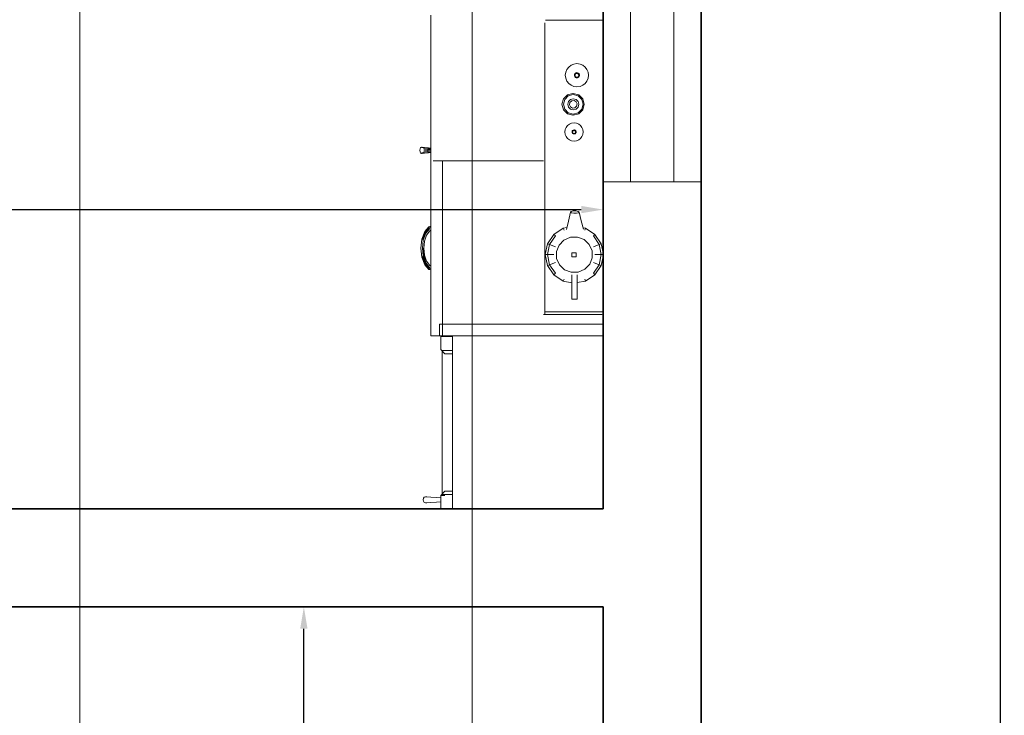
# Model space of a CAD drawing. Units: feet. Extents: x -297 to 770, y -228 to 625.
# Tile 9 of 14: x 680 to 770, y 95 to 158. Entities that reach past the tile are written whole.
import ezdxf

# ---------------------------------------------------------------- set-up
doc = ezdxf.new("R2010")
doc.units = ezdxf.units.FT
doc.header["$MEASUREMENT"] = 0
for name, color, linetype, lineweight in [('A-ANNO-DIMS', 2, 'Continuous', 18), ('A-EQPM', 8, 'Continuous', 13), ('A-FLOR-CASE', 8, 'Continuous', 18), ('A-WALL', 7, 'Continuous', 35), ('windows', 30, 'Continuous', 18)]:
    doc.layers.add(name, color=color, linetype=linetype, lineweight=lineweight)
doc.styles.get("Standard").update_dxf_attribs({"font": 'arial.ttf'})
doc.dimstyles.get("Standard").update_dxf_attribs({"dimtxt": 3, "dimasz": 2, "dimexe": 0.18, "dimexo": 0.0625, "dimgap": 0.09, "dimtad": 1, "dimtoh": 1, "dimdec": 1, "dimzin": 0, "dimdsep": 46, "dimlunit": 3, "dimtxsty": 'Standard', "dimcen": 0, "dimclre": 256, "dimadec": 0, "dimazin": 0, "dimtfac": 1, "dimtdec": 1, "dimtofl": 0, "dimtmove": 0, "dimatfit": 3, "dimfxl": 1, "dimtolj": 1, "dimtzin": 0, "dimlwe": -1, "dimarcsym": 0})

# ---------------------------------------------------------------- blocks, each defined once
blk = doc.blocks.new('WIN-5FT')
for p, q in [((60, 6.5), (0, 6.5)), ((60, 2.5), (0, 2.5))]:
    blk.add_line(p, q)
blk.add_lwpolyline([(60, 0), (60, 9), (0, 9), (0, 0)], close=True)
blk = doc.blocks.new('*D44')
at = {"layer": 'A-ANNO-DIMS', "transparency": 16777216}
for p, q in [((742.218, 306.963), (769.785, 306.963)), ((742.218, -200.037), (769.785, -200.037))]:
    blk.add_line(p, q, dxfattribs=at)
at = {"layer": 'A-ANNO-DIMS', "color": 0, "lineweight": -2, "transparency": 16777216}
blk.add_line((769.605, -198.037), (769.605, 304.963), dxfattribs=at)
at = {"layer": 'A-ANNO-DIMS', "color": 0, "transparency": 16777216}
for points in [[(769.272, 304.963), (769.939, 304.963), (769.605, 306.963)], [(769.272, -198.037), (769.939, -198.037), (769.605, -200.037)]]:
    blk.add_solid(points, dxfattribs=at)
at = {"layer": 'Defpoints', "color": 0, "transparency": 16777216}
for p in [(742.155, 306.963), (769.605, 306.963), (742.155, -200.037)]:
    blk.add_point(p, dxfattribs=at)
at = {"layer": 'A-ANNO-DIMS', "color": 0, "transparency": 16777216, "insert": (767.984, 53.463), "char_height": 3, "attachment_point": 5, "rotation": 90}
blk.add_mtext('\\A1;507', dxfattribs=at)
blk = doc.blocks.new('*D55')
at = {"layer": 'A-ANNO-DIMS', "transparency": 16777216}
for p, q in [((733.093, 104.463), (705.525, 104.463)), ((733.093, 45.463), (705.525, 45.463))]:
    blk.add_line(p, q, dxfattribs=at)
at = {"layer": 'A-ANNO-DIMS', "color": 0, "lineweight": -2, "transparency": 16777216}
blk.add_line((705.705, 47.463), (705.705, 102.463), dxfattribs=at)
at = {"layer": 'A-ANNO-DIMS', "color": 0, "transparency": 16777216}
for points in [[(705.372, 102.463), (706.039, 102.463), (705.705, 104.463)], [(705.372, 47.463), (706.039, 47.463), (705.705, 45.463)]]:
    blk.add_solid(points, dxfattribs=at)
at = {"layer": 'Defpoints', "color": 0, "transparency": 16777216}
for p in [(705.705, 104.463), (733.155, 104.463), (733.155, 45.463)]:
    blk.add_point(p, dxfattribs=at)
at = {"layer": 'A-ANNO-DIMS', "color": 0, "transparency": 16777216, "insert": (704.084, 74.963), "char_height": 3, "attachment_point": 5, "rotation": 90}
blk.add_mtext('\\A1;59', dxfattribs=at)
blk = doc.blocks.new('*D68')
at = {"layer": 'A-ANNO-DIMS', "transparency": 16777216}
for p, q in [((685.155, 306.9), (685.155, -227.667)), ((721.155, 306.9), (721.155, -227.667))]:
    blk.add_line(p, q, dxfattribs=at)
at = {"layer": 'A-ANNO-DIMS', "color": 0, "lineweight": -2, "transparency": 16777216}
blk.add_line((687.155, -227.487), (719.155, -227.487), dxfattribs=at)
at = {"layer": 'A-ANNO-DIMS', "color": 0, "transparency": 16777216}
for points in [[(687.155, -227.154), (687.155, -227.821), (685.155, -227.487)], [(719.155, -227.154), (719.155, -227.821), (721.155, -227.487)]]:
    blk.add_solid(points, dxfattribs=at)
at = {"layer": 'Defpoints', "color": 0, "transparency": 16777216}
for p in [(685.155, 306.963), (721.155, 306.963), (721.155, -227.487)]:
    blk.add_point(p, dxfattribs=at)
at = {"layer": 'A-ANNO-DIMS', "color": 0, "transparency": 16777216, "insert": (703.155, -225.865), "char_height": 3, "attachment_point": 5}
blk.add_mtext('\\A1;36', dxfattribs=at)
blk = doc.blocks.new('*D84')
at = {"layer": 'A-ANNO-DIMS', "transparency": 16777216}
for p, q in [((592.155, 113.525), (592.155, 141.093)), ((733.155, 113.525), (733.155, 141.093))]:
    blk.add_line(p, q, dxfattribs=at)
at = {"layer": 'A-ANNO-DIMS', "color": 0, "lineweight": -2, "transparency": 16777216}
blk.add_line((594.155, 140.913), (731.155, 140.913), dxfattribs=at)
at = {"layer": 'A-ANNO-DIMS', "color": 0, "transparency": 16777216}
for points in [[(594.155, 141.246), (594.155, 140.579), (592.155, 140.913)], [(731.155, 141.246), (731.155, 140.579), (733.155, 140.913)]]:
    blk.add_solid(points, dxfattribs=at)
at = {"layer": 'Defpoints', "color": 0, "transparency": 16777216}
for p in [(733.155, 140.913), (592.155, 113.463), (733.155, 113.463)]:
    blk.add_point(p, dxfattribs=at)
at = {"layer": 'A-ANNO-DIMS', "color": 0, "transparency": 16777216, "insert": (662.655, 142.509), "char_height": 3, "attachment_point": 5}
blk.add_mtext('\\A1;141', dxfattribs=at)

msp = doc.modelspace()

# ---------------------------------------------------------------- linework, layer by layer
at = {"layer": 'A-EQPM'}
for p, q in [((727.797, 131.305), (727.797, 158.049)), ((729.832, 153.777), (729.724, 153.523)), ((729.999, 153.993), (729.832, 153.777)), ((730.215, 154.16), (729.999, 153.993)), ((730.47, 154.268), (730.215, 154.16)), ((730.753, 154.306), (730.47, 154.268)), ((731.036, 154.268), (730.753, 154.306)), ((731.291, 154.16), (731.036, 154.268)), ((731.507, 153.993), (731.291, 154.16)), ((731.674, 153.777), (731.507, 153.993)), ((731.781, 153.523), (731.674, 153.777)), ((729.724, 153.523), (729.686, 153.239)), ((729.686, 153.239), (729.724, 152.956)), ((729.724, 152.956), (729.832, 152.701)), ((729.832, 152.701), (729.999, 152.485)), ((730.526, 153.302), (730.517, 153.239)), ((730.517, 153.239), (730.526, 153.177)), ((730.55, 153.358), (730.526, 153.302)), ((730.526, 153.177), (730.55, 153.12)), ((730.544, 153.297), (730.536, 153.239)), ((730.536, 153.239), (730.544, 153.181)), ((730.566, 153.349), (730.544, 153.297)), ((730.544, 153.181), (730.566, 153.13)), ((730.586, 153.406), (730.55, 153.358)), ((730.55, 153.12), (730.586, 153.073)), ((730.6, 153.393), (730.566, 153.349)), ((730.566, 153.13), (730.6, 153.086)), ((730.58, 153.276), (730.574, 153.229)), ((730.574, 153.229), (730.58, 153.181)), ((730.598, 153.319), (730.58, 153.276)), ((730.58, 153.181), (730.598, 153.139)), ((730.634, 153.443), (730.586, 153.406)), ((730.586, 153.073), (730.634, 153.036)), ((730.626, 153.355), (730.598, 153.319)), ((730.598, 153.139), (730.626, 153.102)), ((730.643, 153.426), (730.6, 153.393)), ((730.6, 153.086), (730.643, 153.052)), ((730.663, 153.383), (730.626, 153.355)), ((730.626, 153.102), (730.663, 153.074)), ((730.69, 153.466), (730.634, 153.443)), ((730.634, 153.036), (730.69, 153.012)), ((730.695, 153.448), (730.643, 153.426)), ((730.643, 153.052), (730.695, 153.03)), ((730.705, 153.401), (730.663, 153.383)), ((730.663, 153.074), (730.705, 153.056)), ((730.753, 153.475), (730.69, 153.466)), ((730.69, 153.012), (730.753, 153.003)), ((730.753, 153.456), (730.695, 153.448)), ((730.695, 153.03), (730.753, 153.022)), ((730.753, 153.408), (730.705, 153.401)), ((730.705, 153.056), (730.753, 153.05)), ((730.816, 153.466), (730.753, 153.475)), ((730.811, 153.448), (730.753, 153.456)), ((730.8, 153.401), (730.753, 153.408)), ((730.753, 153.05), (730.8, 153.056)), ((730.753, 153.022), (730.811, 153.03)), ((730.753, 153.003), (730.816, 153.012)), ((730.843, 153.383), (730.8, 153.401)), ((730.8, 153.056), (730.843, 153.074)), ((730.862, 153.426), (730.811, 153.448)), ((730.811, 153.03), (730.862, 153.052)), ((730.872, 153.443), (730.816, 153.466)), ((730.816, 153.012), (730.872, 153.036)), ((730.879, 153.355), (730.843, 153.383)), ((730.843, 153.074), (730.879, 153.102)), ((730.906, 153.393), (730.862, 153.426)), ((730.862, 153.052), (730.906, 153.086)), ((730.919, 153.406), (730.872, 153.443)), ((730.872, 153.036), (730.919, 153.073)), ((730.907, 153.319), (730.879, 153.355)), ((730.879, 153.102), (730.907, 153.139)), ((730.94, 153.349), (730.906, 153.393)), ((730.906, 153.086), (730.94, 153.13)), ((730.926, 153.276), (730.907, 153.319)), ((730.907, 153.139), (730.926, 153.181)), ((730.956, 153.358), (730.919, 153.406)), ((730.919, 153.073), (730.956, 153.12)), ((730.932, 153.229), (730.926, 153.276)), ((730.926, 153.181), (730.932, 153.229)), ((730.962, 153.297), (730.94, 153.349)), ((730.94, 153.13), (730.962, 153.181)), ((730.98, 153.302), (730.956, 153.358)), ((730.956, 153.12), (730.98, 153.177)), ((730.97, 153.239), (730.962, 153.297)), ((730.962, 153.181), (730.97, 153.239)), ((730.989, 153.239), (730.98, 153.302)), ((730.98, 153.177), (730.989, 153.239)), ((731.507, 152.485), (731.674, 152.701)), ((731.674, 152.701), (731.781, 152.956)), ((731.82, 153.239), (731.781, 153.523)), ((731.781, 152.956), (731.82, 153.239)), ((729.999, 152.485), (730.215, 152.318)), ((730.215, 152.318), (730.47, 152.21)), ((730.47, 152.21), (730.753, 152.172)), ((730.753, 152.172), (731.036, 152.21)), ((731.036, 152.21), (731.291, 152.318)), ((731.291, 152.318), (731.507, 152.485)), ((729.521, 151.079), (729.383, 150.571)), ((729.635, 151.027), (729.511, 150.57)), ((729.882, 151.441), (729.521, 151.079)), ((729.96, 151.352), (729.635, 151.027)), ((730.39, 151.578), (729.882, 151.441)), ((729.978, 150.827), (729.908, 150.57)), ((730.417, 151.476), (729.96, 151.352)), ((730.161, 151.009), (729.978, 150.827)), ((730.109, 150.746), (730.272, 150.893)), ((730.417, 151.079), (730.161, 151.009)), ((730.272, 150.893), (730.49, 150.916)), ((730.389, 151.568), (730.39, 151.578)), ((730.389, 151.569), (730.417, 151.577)), ((730.417, 151.577), (730.925, 151.439)), ((730.874, 151.352), (730.417, 151.476)), ((730.674, 151.009), (730.417, 151.079)), ((730.49, 150.916), (730.681, 150.807)), ((730.856, 150.827), (730.674, 151.009)), ((730.926, 150.57), (730.856, 150.827)), ((731.199, 151.027), (730.874, 151.352)), ((730.925, 151.439), (731.286, 151.078)), ((731.323, 150.57), (731.199, 151.027)), ((731.286, 151.078), (731.424, 150.57)), ((729.383, 150.571), (729.521, 150.063)), ((729.511, 150.57), (729.635, 150.113)), ((729.521, 150.063), (729.882, 149.702)), ((729.635, 150.113), (729.96, 149.788)), ((729.908, 150.57), (729.978, 150.313)), ((729.978, 150.313), (730.161, 150.131)), ((730.064, 150.53), (730.109, 150.746)), ((730.153, 150.33), (730.064, 150.53)), ((730.344, 150.22), (730.153, 150.33)), ((730.161, 150.131), (730.417, 150.061)), ((730.562, 150.244), (730.344, 150.22)), ((730.417, 150.061), (730.674, 150.131)), ((730.725, 150.391), (730.562, 150.244)), ((730.674, 150.131), (730.856, 150.313)), ((730.681, 150.807), (730.771, 150.606)), ((730.771, 150.606), (730.725, 150.391)), ((730.856, 150.313), (730.926, 150.57)), ((730.874, 149.788), (731.199, 150.113)), ((731.286, 150.062), (730.925, 149.701)), ((731.199, 150.113), (731.323, 150.57)), ((731.424, 150.57), (731.286, 150.062)), ((729.882, 149.702), (730.39, 149.564)), ((729.96, 149.788), (730.417, 149.664)), ((730.39, 149.564), (730.389, 149.572)), ((730.417, 149.563), (730.389, 149.571)), ((730.417, 149.664), (730.874, 149.788)), ((730.925, 149.701), (730.417, 149.563)), ((729.681, 148.257), (729.651, 148.034)), ((729.766, 148.457), (729.681, 148.257)), ((729.897, 148.627), (729.766, 148.457)), ((730.067, 148.759), (729.897, 148.627)), ((730.268, 148.843), (730.067, 148.759)), ((730.491, 148.873), (730.268, 148.843)), ((730.33, 148.127), (730.312, 148.083)), ((730.343, 148.12), (730.326, 148.079)), ((730.359, 148.165), (730.33, 148.127)), ((730.37, 148.154), (730.343, 148.12)), ((730.397, 148.194), (730.359, 148.165)), ((730.391, 148.125), (730.369, 148.097)), ((730.404, 148.181), (730.37, 148.154)), ((730.419, 148.147), (730.391, 148.125)), ((730.441, 148.213), (730.397, 148.194)), ((730.445, 148.198), (730.404, 148.181)), ((730.453, 148.162), (730.419, 148.147)), ((730.491, 148.219), (730.441, 148.213)), ((730.491, 148.205), (730.445, 148.198)), ((730.491, 148.167), (730.453, 148.162)), ((730.713, 148.843), (730.491, 148.873)), ((730.54, 148.213), (730.491, 148.219)), ((730.536, 148.198), (730.491, 148.205)), ((730.528, 148.162), (730.491, 148.167)), ((730.562, 148.147), (730.528, 148.162)), ((730.577, 148.181), (730.536, 148.198)), ((730.584, 148.194), (730.54, 148.213)), ((730.59, 148.125), (730.562, 148.147)), ((730.611, 148.154), (730.577, 148.181)), ((730.622, 148.165), (730.584, 148.194)), ((730.612, 148.097), (730.59, 148.125)), ((730.638, 148.12), (730.611, 148.154)), ((730.651, 148.127), (730.622, 148.165)), ((730.655, 148.079), (730.638, 148.12)), ((730.669, 148.083), (730.651, 148.127)), ((730.914, 148.759), (730.713, 148.843)), ((731.084, 148.627), (730.914, 148.759)), ((731.215, 148.457), (731.084, 148.627)), ((731.3, 148.257), (731.215, 148.457)), ((731.33, 148.034), (731.3, 148.257)), ((729.651, 148.034), (729.681, 147.811)), ((729.681, 147.811), (729.766, 147.61)), ((729.766, 147.61), (729.897, 147.44)), ((729.897, 147.44), (730.067, 147.309)), ((730.067, 147.309), (730.268, 147.224)), ((730.268, 147.224), (730.491, 147.194)), ((730.312, 148.083), (730.305, 148.034)), ((730.305, 148.034), (730.312, 147.984)), ((730.312, 147.984), (730.33, 147.94)), ((730.326, 148.079), (730.32, 148.034)), ((730.32, 148.034), (730.326, 147.988)), ((730.326, 147.988), (730.343, 147.948)), ((730.33, 147.94), (730.359, 147.903)), ((730.343, 147.948), (730.37, 147.913)), ((730.355, 148.063), (730.35, 148.026)), ((730.35, 148.026), (730.355, 147.988)), ((730.369, 148.097), (730.355, 148.063)), ((730.355, 147.988), (730.369, 147.955)), ((730.359, 147.903), (730.397, 147.874)), ((730.369, 147.955), (730.391, 147.926)), ((730.37, 147.913), (730.404, 147.886)), ((730.391, 147.926), (730.419, 147.904)), ((730.397, 147.874), (730.441, 147.855)), ((730.404, 147.886), (730.445, 147.869)), ((730.419, 147.904), (730.453, 147.89)), ((730.441, 147.855), (730.491, 147.848)), ((730.445, 147.869), (730.491, 147.863)), ((730.453, 147.89), (730.491, 147.885)), ((730.491, 147.885), (730.528, 147.89)), ((730.491, 147.863), (730.536, 147.869)), ((730.491, 147.848), (730.54, 147.855)), ((730.491, 147.194), (730.713, 147.224)), ((730.528, 147.89), (730.562, 147.904)), ((730.536, 147.869), (730.577, 147.886)), ((730.54, 147.855), (730.584, 147.874)), ((730.562, 147.904), (730.59, 147.926)), ((730.577, 147.886), (730.611, 147.913)), ((730.584, 147.874), (730.622, 147.903)), ((730.59, 147.926), (730.612, 147.955)), ((730.611, 147.913), (730.638, 147.948)), ((730.626, 148.063), (730.612, 148.097)), ((730.612, 147.955), (730.626, 147.988)), ((730.622, 147.903), (730.651, 147.94)), ((730.631, 148.026), (730.626, 148.063)), ((730.626, 147.988), (730.631, 148.026)), ((730.638, 147.948), (730.655, 147.988)), ((730.651, 147.94), (730.669, 147.984)), ((730.661, 148.034), (730.655, 148.079)), ((730.655, 147.988), (730.661, 148.034)), ((730.676, 148.034), (730.669, 148.083)), ((730.669, 147.984), (730.676, 148.034)), ((730.713, 147.224), (730.914, 147.309)), ((730.914, 147.309), (731.084, 147.44)), ((731.084, 147.44), (731.215, 147.61)), ((731.215, 147.61), (731.3, 147.811)), ((731.3, 147.811), (731.33, 148.034)), ((729.966, 139.838), (730.175, 140.67)), ((730.175, 140.67), (730.234, 140.737)), ((730.264, 140.613), (730.175, 140.67)), ((730.234, 140.737), (730.417, 140.787)), ((730.465, 140.582), (730.264, 140.613)), ((730.417, 140.787), (730.654, 140.793)), ((730.703, 140.586), (730.465, 140.582)), ((730.654, 140.793), (730.856, 140.751)), ((730.886, 140.623), (730.703, 140.586)), ((730.856, 140.751), (730.944, 140.684)), ((730.944, 140.684), (730.886, 140.623)), ((730.944, 140.684), (731.153, 139.867)), ((728.629, 138.633), (729.496, 139.201)), ((729.496, 139.201), (729.828, 139.266)), ((729.496, 139.201), (729.574, 139.017)), ((729.787, 139.1), (729.966, 139.838)), ((731.153, 139.867), (731.341, 139.106)), ((731.306, 139.248), (731.543, 139.201)), ((731.543, 139.201), (731.465, 139.017)), ((731.543, 139.201), (732.41, 138.633)), ((728.049, 137.783), (728.629, 138.633)), ((728.773, 138.492), (728.238, 137.707)), ((728.629, 138.633), (728.773, 138.492)), ((730.158, 138.379), (729.562, 138.121)), ((730.81, 138.393), (730.158, 138.379)), ((731.417, 138.161), (730.81, 138.393)), ((732.41, 138.633), (732.266, 138.492)), ((732.266, 138.492), (732.802, 137.707)), ((732.41, 138.633), (732.99, 137.783)), ((727.846, 136.781), (728.049, 137.783)), ((728.049, 137.783), (728.238, 137.707)), ((728.238, 137.707), (728.049, 136.781)), ((728.238, 137.707), (728.773, 137.49)), ((729.111, 137.66), (728.875, 137.065)), ((729.562, 138.121), (729.111, 137.66)), ((731.888, 137.719), (731.417, 138.161)), ((732.15, 137.135), (731.888, 137.719)), ((732.802, 137.707), (732.266, 137.49)), ((732.99, 137.783), (732.802, 137.707)), ((732.802, 137.707), (732.99, 136.781)), ((732.99, 137.783), (733.158, 136.955)), ((728.049, 136.781), (727.846, 136.781)), ((727.846, 136.781), (728.049, 135.778)), ((728.049, 136.781), (728.629, 136.781)), ((728.238, 135.854), (728.049, 136.781)), ((728.875, 137.065), (728.889, 136.426)), ((728.889, 136.426), (729.152, 135.842)), ((730.299, 136.945), (730.685, 136.945)), ((730.299, 136.566), (730.299, 136.945)), ((730.685, 136.566), (730.299, 136.566)), ((730.685, 136.945), (730.685, 136.566)), ((731.928, 135.901), (732.164, 136.496)), ((732.164, 136.496), (732.15, 137.135)), ((732.99, 136.781), (732.41, 136.781)), ((732.802, 135.854), (732.99, 136.781)), ((732.99, 136.781), (733.158, 136.781)), ((732.99, 135.778), (733.158, 136.607)), ((728.049, 135.778), (728.238, 135.854)), ((728.049, 135.778), (728.629, 134.928)), ((728.238, 135.854), (728.773, 136.072)), ((728.773, 135.069), (728.238, 135.854)), ((729.152, 135.842), (729.622, 135.4)), ((731.478, 135.44), (731.928, 135.901)), ((732.802, 135.854), (732.266, 136.072)), ((732.266, 135.069), (732.802, 135.854)), ((732.41, 134.928), (732.99, 135.778)), ((732.99, 135.778), (732.802, 135.854)), ((728.629, 134.928), (728.773, 135.069)), ((728.629, 134.928), (729.496, 134.36)), ((729.622, 135.4), (730.23, 135.169)), ((730.23, 135.169), (730.881, 135.183)), ((730.287, 132.709), (730.287, 134.934)), ((730.782, 134.938), (730.782, 134.766)), ((730.782, 134.766), (730.782, 134.627)), ((730.782, 134.627), (730.782, 134.368)), ((730.881, 135.183), (731.478, 135.44)), ((731.543, 134.36), (732.41, 134.928)), ((732.41, 134.928), (732.266, 135.069)), ((729.496, 134.36), (729.574, 134.544)), ((729.496, 134.36), (730.287, 134.206)), ((730.782, 134.368), (730.782, 133.913)), ((730.782, 134.211), (731.543, 134.36)), ((730.782, 133.913), (730.782, 133.454)), ((731.543, 134.36), (731.465, 134.544)), ((730.782, 133.454), (730.782, 133.07)), ((730.782, 133.07), (730.782, 132.817)), ((730.782, 132.817), (730.782, 132.709)), ((730.782, 132.709), (730.287, 132.709)), ((733.047, 131.274), (727.699, 131.274)), ((733.158, 131.54), (727.858, 131.54)), ((733.047, 131.305), (733.047, 131.274))]:
    msp.add_line(p, q, dxfattribs=at)
at = {"layer": 'A-FLOR-CASE'}
for p, q in [((733.155, 113.516), (733.155, 233.463)), ((717.346, 145.385), (717.346, 158.757)), ((727.858, 158.285), (733.158, 158.285)), ((716.36, 146.501), (716.341, 146.355)), ((716.341, 146.355), (716.36, 146.208)), ((716.412, 146.608), (716.36, 146.501)), ((716.484, 146.647), (716.412, 146.608)), ((716.562, 146.639), (716.484, 146.647)), ((716.498, 146.601), (716.742, 146.581)), ((716.787, 146.616), (716.562, 146.639)), ((717.083, 146.355), (716.697, 146.355)), ((716.742, 146.581), (716.709, 146.485)), ((716.709, 146.485), (717.088, 146.466)), ((716.742, 146.581), (716.787, 146.616)), ((717.103, 146.547), (716.742, 146.581)), ((716.787, 146.616), (717.124, 146.577)), ((717.088, 146.466), (717.083, 146.355)), ((717.346, 146.355), (717.083, 146.355)), ((717.083, 146.355), (717.088, 146.244)), ((717.088, 146.466), (717.103, 146.547)), ((717.346, 146.449), (717.088, 146.466)), ((717.124, 146.577), (717.103, 146.547)), ((717.103, 146.547), (717.346, 146.519)), ((717.124, 146.577), (717.346, 146.546)), ((716.36, 146.208), (716.412, 146.101)), ((716.412, 146.101), (716.484, 146.062)), ((716.484, 146.062), (716.562, 146.07)), ((716.742, 146.129), (716.498, 146.108)), ((716.562, 146.07), (716.787, 146.094)), ((717.088, 146.244), (716.709, 146.224)), ((716.709, 146.224), (716.742, 146.129)), ((716.742, 146.129), (717.103, 146.162)), ((716.787, 146.094), (716.742, 146.129)), ((716.787, 146.094), (717.124, 146.133)), ((717.088, 146.244), (717.346, 146.26)), ((717.103, 146.162), (717.088, 146.244)), ((717.103, 146.162), (717.346, 146.19)), ((717.124, 146.133), (717.103, 146.162)), ((717.124, 146.133), (717.346, 146.163)), ((717.346, 129.343), (717.346, 145.385)), ((717.576, 145.375), (727.699, 145.375)), ((718.174, 145.376), (727.699, 145.375)), ((718.416, 145.385), (718.416, 129.343)), ((727.699, 145.376), (719.378, 145.377)), ((719.378, 145.377), (719.379, 145.376)), ((716.789, 138.906), (717.175, 139.341)), ((717.18, 139.317), (716.801, 138.884)), ((716.834, 138.823), (717.195, 139.249)), ((717.216, 139.156), (716.879, 138.739)), ((717.175, 139.341), (717.346, 139.385)), ((717.175, 139.341), (717.18, 139.317)), ((717.346, 139.361), (717.18, 139.317)), ((717.18, 139.317), (717.195, 139.249)), ((717.195, 139.249), (717.346, 139.295)), ((717.195, 139.249), (717.216, 139.156)), ((716.433, 137.379), (716.526, 138.214)), ((716.526, 138.214), (716.789, 138.906)), ((716.834, 138.823), (716.59, 138.164)), ((716.654, 138.115), (716.879, 138.739)), ((716.783, 138.017), (716.969, 138.572)), ((716.801, 138.884), (716.834, 138.823)), ((716.879, 138.739), (716.834, 138.823)), ((716.969, 138.572), (717.258, 138.971)), ((717.258, 138.971), (717.346, 139.016)), ((716.526, 136.545), (716.433, 137.379)), ((716.575, 137.379), (716.654, 138.115)), ((716.654, 136.643), (716.575, 137.379)), ((716.647, 137.379), (716.718, 136.692)), ((716.718, 137.379), (716.783, 138.017)), ((716.783, 136.742), (716.718, 137.379)), ((716.789, 135.852), (716.526, 136.545)), ((716.59, 136.594), (716.834, 135.936)), ((716.654, 136.643), (716.718, 136.692)), ((716.879, 136.019), (716.654, 136.643)), ((716.718, 136.692), (716.765, 136.728)), ((716.718, 136.692), (716.879, 136.019)), ((716.969, 136.186), (716.783, 136.742)), ((717.175, 135.417), (716.789, 135.852)), ((716.834, 135.936), (716.801, 135.875)), ((716.801, 135.875), (717.18, 135.442)), ((716.879, 136.019), (716.834, 135.936)), ((716.834, 135.936), (717.195, 135.509)), ((717.216, 135.602), (716.879, 136.019)), ((717.258, 135.787), (716.969, 136.186)), ((717.18, 135.442), (717.195, 135.509)), ((717.195, 135.509), (717.216, 135.602)), ((717.195, 135.509), (717.346, 135.463)), ((717.346, 135.743), (717.258, 135.787)), ((717.175, 135.417), (717.18, 135.442)), ((717.346, 135.373), (717.175, 135.417)), ((717.18, 135.442), (717.346, 135.397)), ((718.148, 130.413), (733.155, 130.413)), ((718.148, 129.343), (718.148, 130.413)), ((718.416, 129.343), (717.346, 129.343)), ((733.155, 129.343), (718.148, 129.343)), ((718.278, 129.272), (719.325, 129.272)), ((718.278, 128.069), (718.278, 129.272)), ((719.325, 113.487), (719.325, 129.343)), ((718.627, 127.668), (718.278, 128.069)), ((718.404, 127.989), (719.325, 127.989)), ((718.404, 114.77), (718.404, 127.989)), ((719.325, 127.668), (718.627, 127.668)), ((718.278, 114.69), (718.627, 115.091)), ((719.325, 114.77), (718.404, 114.77)), ((718.627, 115.091), (719.325, 115.091)), ((716.639, 114.289), (716.669, 114.429)), ((716.669, 114.149), (716.639, 114.289)), ((716.669, 114.429), (716.75, 114.532)), ((716.75, 114.046), (716.669, 114.149)), ((716.75, 114.532), (716.862, 114.57)), ((716.862, 114.008), (716.75, 114.046)), ((716.862, 114.57), (716.986, 114.562)), ((716.986, 114.016), (716.862, 114.008)), ((716.986, 114.562), (717.338, 114.54)), ((717.338, 114.038), (716.986, 114.016)), ((717.338, 114.54), (717.865, 114.502)), ((717.338, 114.038), (717.865, 114.076)), ((717.865, 114.502), (718.278, 114.467)), ((717.865, 114.076), (718.278, 114.111)), ((718.278, 114.69), (718.627, 114.69)), ((718.278, 114.289), (718.278, 114.69)), ((718.278, 113.487), (718.278, 114.289)), ((719.325, 113.487), (718.278, 113.487)), ((733.155, 113.487), (719.325, 113.487))]:
    msp.add_line(p, q, dxfattribs=at)
at = {"layer": 'A-WALL'}
for p, q in [((742.155, -200.037), (742.155, 306.963)), ((733.155, 113.463), (648.155, 113.463)), ((733.155, 104.463), (648.155, 104.463))]:
    msp.add_line(p, q, dxfattribs=at)
for points in [[(733.155, 113.463), (733.155, 233.463)], [(733.155, -63.537), (733.155, 104.463)]]:
    msp.add_lwpolyline(points, dxfattribs=at)

# ---------------------------------------------------------------- block references
at = {"layer": 'windows', "rotation": 90.00000000000003}
msp.add_blockref('WIN-5FT', (742.155, 143.463), dxfattribs=at)

# ---------------------------------------------------------------- dimensions: what is measured, and where the dimension line sits
at = {"layer": 'A-ANNO-DIMS'}
for base, p1, p2, picture, middle in [((721.155, -227.487), (685.155, 306.963), (721.155, 306.963), '*D68', (703.155, -225.865)), ((733.155, 140.913), (592.155, 113.463), (733.155, 113.463), '*D84', (662.655, 142.509))]:
    dim = msp.add_linear_dim(base=base, p1=p1, p2=p2, dimstyle='Standard', override={"dimdec": 0, "dimlfac": 1, "dimrnd": 0, "dimzin": 0, "dimdsep": 46, "dimlunit": 2}, dxfattribs=at)
    dim.commit()
    dim.dimension.update_dxf_attribs({"geometry": picture, "text_midpoint": middle})
for base, p1, p2, picture, middle in [((769.605, 306.963), (742.155, -200.037), (742.155, 306.963), '*D44', (767.984, 53.463)), ((705.705, 104.463), (733.155, 45.463), (733.155, 104.463), '*D55', (704.084, 74.963))]:
    dim = msp.add_linear_dim(base=base, p1=p1, p2=p2, angle=90, dimstyle='Standard', override={"dimdec": 0, "dimlfac": 1, "dimrnd": 0, "dimzin": 0, "dimdsep": 46, "dimlunit": 2}, dxfattribs=at)
    dim.commit()
    dim.dimension.update_dxf_attribs({"geometry": picture, "text_midpoint": middle})

doc.saveas('drawing.dxf')
